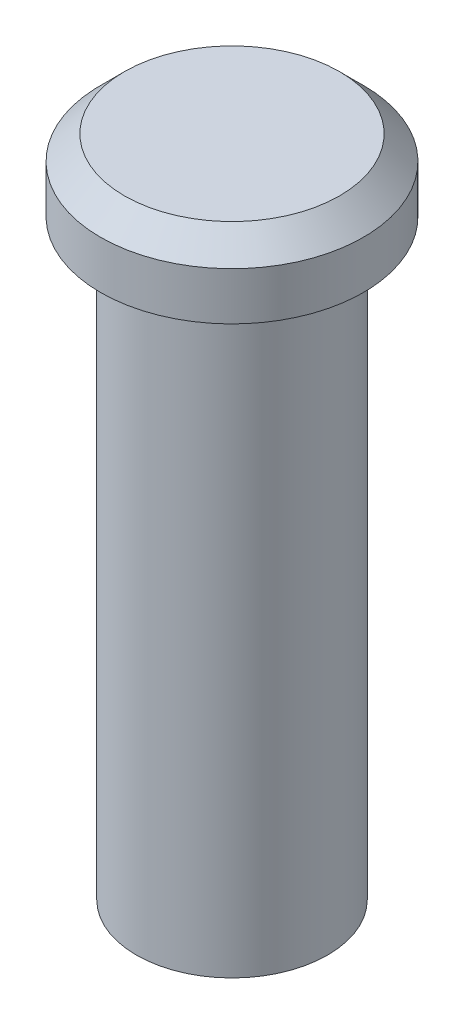
from build123d import *

# Parameters (mm, degrees)
SHANK_PROFILE_8_R      = 4
SHANK_8_DEPTH          = 24.75
HEAD_PROFILE_14_R      = 5.5
HEAD_14_DEPTH          = 3
HEAD_CHAMFER_1X45_SIZE = 1


with BuildPart() as part:
    # Shank Profile Ø8 → Shank Ø8 (new body)
    with BuildSketch(Plane(origin=(0, 0, 0), x_dir=(1, 0, 0), z_dir=(0, 1, 0))):
        with Locations(Location((0, 0, 0), (0, 0, 270))):
            Circle(SHANK_PROFILE_8_R)
    extrude(amount=SHANK_8_DEPTH)

    # Head Profile Ø14 → Head Ø14 (add)
    with BuildSketch(Plane(origin=(0, 24.75, 0), x_dir=(1, 0, 0), z_dir=(0, 1, 0))):
        with Locations(Location((0, 0, 0), (0, 0, 270))):
            Circle(HEAD_PROFILE_14_R)
    extrude(amount=HEAD_14_DEPTH)

    # Head Chamfer 1x45°
    head_chamfer_1x45_edges = [part.edges().sort_by_distance(p)[0] for p in [
        (0, 27.75, -5.5),
    ]]
    chamfer(head_chamfer_1x45_edges, length=HEAD_CHAMFER_1X45_SIZE)


solid = part.part
